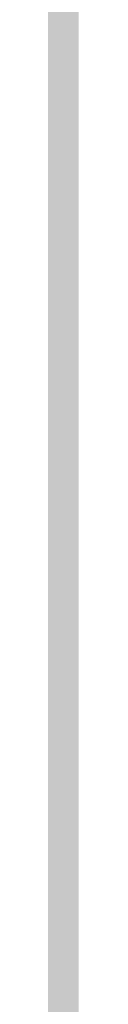
# Model space of a CAD drawing. Units: inches. Extents: x 2083 to 3317, y 1141 to 2115.
# Tile 181 of 256: x 3126.95825 to 3126.9594, y 1263.29018 to 1263.35483. Entities that reach past the tile are written whole.
import ezdxf

# ---------------------------------------------------------------- set-up
doc = ezdxf.new("R2010")
doc.units = ezdxf.units.IN
doc.layers.add('A-ANNO-DIMS', color=2, linetype='Continuous', lineweight=18)
doc.layers.add('A-WALL-PATT', color=251, linetype='Continuous', lineweight=13, true_color=0x636466)
doc.styles.get("Standard").update_dxf_attribs({"font": 'arial.ttf'})
doc.dimstyles.new('ISO-25', dxfattribs={"dimtxt": 12, "dimasz": 12, "dimexe": 1.25, "dimexo": 0.625, "dimtad": 1, "dimlunit": 3, "dimtxsty": 'Standard', "dimcen": 2.5, "dimadec": 0, "dimazin": 0, "dimtfac": 1, "dimtmove": 0, "dimatfit": 3, "dimfxl": 1, "dimarcsym": 0})

# ---------------------------------------------------------------- blocks, each defined once
blk = doc.blocks.new('*D26')
at = {"layer": 'A-ANNO-DIMS', "color": 0, "lineweight": -2, "transparency": 16777216}
for p, q in [((3088.985844, 1274.915092), (3088.985844, 1270.951963)), ((3111.240037, 1274.915092), (3111.240037, 1270.951963)), ((3076.985844, 1272.201963), (2840.262447, 1272.201963)), ((3111.240037, 1272.201963), (3088.985844, 1272.201963)), ((3123.240037, 1272.201963), (3135.240037, 1272.201963))]:
    blk.add_line(p, q, dxfattribs=at)
at = {"layer": 'A-ANNO-DIMS', "color": 0, "transparency": 16777216}
for points in [[(3076.985844, 1274.201963), (3076.985844, 1270.201963), (3088.985844, 1272.201963)], [(3123.240037, 1274.201963), (3123.240037, 1270.201963), (3111.240037, 1272.201963)]]:
    blk.add_solid(points, dxfattribs=at)
at = {"layer": 'Defpoints', "color": 0, "transparency": 16777216}
for p in [(3088.985844, 1275.540092), (3111.240037, 1275.540092), (3088.985844, 1272.201963)]:
    blk.add_point(p, dxfattribs=at)
at = {"layer": 'A-ANNO-DIMS', "color": 0, "transparency": 16777216, "insert": (2952.624146, 1279.031602), "char_height": 12, "attachment_point": 5}
blk.add_mtext('NIGHTSTAND 1\'-10 1/2" TYP.', dxfattribs=at)
blk = doc.blocks.new('*D27')
at = {"layer": 'A-ANNO-DIMS', "color": 0, "lineweight": -2, "transparency": 16777216}
for p, q in [((3114.578165, 1309.794285), (3114.578165, 1321.794285)), ((3111.865037, 1297.794285), (3115.828165, 1297.794285)), ((3114.578165, 1297.794285), (3114.578165, 1275.540092)), ((3111.865037, 1275.540092), (3115.828165, 1275.540092)), ((3114.578165, 1263.540092), (3114.578165, 1140.988591))]:
    blk.add_line(p, q, dxfattribs=at)
at = {"layer": 'A-ANNO-DIMS', "color": 0, "transparency": 16777216}
for points in [[(3112.578165, 1309.794285), (3116.578165, 1309.794285), (3114.578165, 1297.794285)], [(3112.578165, 1263.540092), (3116.578165, 1263.540092), (3114.578165, 1275.540092)]]:
    blk.add_solid(points, dxfattribs=at)
at = {"layer": 'Defpoints', "color": 0, "transparency": 16777216}
for p in [(3111.240037, 1297.794285), (3111.240037, 1275.540092), (3114.578165, 1275.540092)]:
    blk.add_point(p, dxfattribs=at)
at = {"layer": 'A-ANNO-DIMS', "color": 0, "transparency": 16777216, "insert": (3107.748527, 1196.264342), "char_height": 12, "attachment_point": 5, "rotation": 90}
blk.add_mtext('1\'-10 1/2" TYP.', dxfattribs=at)

msp = doc.modelspace()

# ---------------------------------------------------------------- hatches: boundary and pattern name
at = {"layer": 'A-WALL-PATT'}
h = msp.add_hatch(color=256, dxfattribs=at)
h.dxf.hatch_style = 1
h.paths.add_polyline_path([(3126.959783, 2020.76136), (2748.959783, 2020.76136), (2604.959783, 2020.76136), (2226.959783, 2020.76136), (2226.959783, 1702.76136), (2466.959783, 1702.76136), (2466.959783, 1582.76136), (2418.959783, 1582.76136), (2418.959783, 1477.76136), (2226.959783, 1477.76136), (2226.959783, 1263.26136), (2544.959783, 1263.26136), (2544.959783, 1411.76136), (2604.959783, 1411.76136), (2685.959783, 1411.76136), (2685.959783, 1420.76136), (2604.959783, 1420.76136), (2604.959783, 1573.76136), (2604.959783, 1702.76136), (2604.959783, 2011.76136), (2748.959783, 2011.76136), (2748.959783, 1702.76136), (2862.959783, 1702.76136), (2862.959783, 1621.76136), (2871.959783, 1621.76136), (2871.959783, 1702.76136), (2883.959783, 1702.76136), (2883.959783, 1706.939459, -0.026459), (2883.959783, 1711.76136), (2757.959783, 1711.76136), (2757.959783, 1807.76136), (2787.959783, 1807.76136), (2787.959783, 1812.26136), (2757.959783, 1812.26136), (2757.959783, 2011.76136), (2877.959783, 2011.76136), (2877.959783, 1812.26136), (2847.959783, 1812.26136), (2847.959783, 1807.76136), (2889.835742, 1807.76136), (2889.835742, 1812.26136), (2882.459783, 1812.26136), (2882.459783, 2011.76136), (3117.959783, 2011.76136), (3117.959783, 1812.26136), (2937.835742, 1812.26136), (2937.835742, 1807.76136), (2995.709783, 1807.76136), (2995.709783, 1796.117666), (3000.209783, 1796.117666), (3000.209783, 1807.76136), (3117.959783, 1807.76136), (3117.959783, 1711.76136), (3000.209783, 1711.76136), (3000.209783, 1760.117666), (2998.572705, 1760.117666, -0.020711), (2995.709783, 1760.117666), (2995.709783, 1711.76136), (2931.959783, 1711.76136), (2931.959783, 1702.76136), (3126.959783, 1702.76136)])
h.paths.add_polyline_path([(2471.459783, 2011.76136), (2471.459783, 1810.01136), (2462.716936, 1810.01136), (2462.716936, 1805.51136), (2505.959783, 1805.51136), (2505.959783, 1810.01136), (2475.959783, 1810.01136), (2475.959783, 2011.76136), (2595.959783, 2011.76136), (2595.959783, 1810.01136), (2565.959783, 1810.01136), (2565.959783, 1805.51136), (2595.959783, 1805.51136), (2595.959783, 1711.76136), (2235.959783, 1711.76136), (2235.959783, 1805.51136), (2353.709783, 1805.51136), (2353.709783, 1796.054162), (2358.209783, 1796.054162), (2358.209783, 1805.51136), (2414.716936, 1805.51136), (2414.716936, 1810.01136), (2235.959783, 1810.01136), (2235.959783, 2011.76136)], flags=16)
h.paths.add_polyline_path([(2270.204734, 1994.610008), (2270.204734, 1970.610008), (2246.204734, 1970.610008), (2246.204734, 1994.610008)], flags=0)
edge = h.paths.add_edge_path(flags=0)
edge.add_ellipse((2332.027391, 1899.798176), major_axis=(-3.042994, 3.042994), ratio=0.16825245, start_angle=-161.332166, end_angle=-156.307114, ccw=False)
edge.add_ellipse((2333.082037, 1898.74353), major_axis=(-1.054646, 1.054646), ratio=0.4535321, start_angle=-123.371019, end_angle=-94.159107)
edge = h.paths.add_edge_path(flags=0)
edge.add_ellipse((2332.027391, 1968.87629), major_axis=(3.042994, 3.042994), ratio=0.16825245, start_angle=18.667834, end_angle=23.692886)
edge.add_spline(control_points=[(2332.925596, 1970.691105), (2332.226768, 1970.3361), (2330.893709, 1969.658905), (2328.41308, 1970.932138), (2327.203934, 1967.748712), (2324.709596, 1969.955589), (2322.532822, 1967.012354), (2320.012846, 1971.295812), (2317.680308, 1968.157845), (2316.040526, 1967.102047), (2315.426904, 1966.809602)], knot_values=[0, 0, 0, 0, 2.267059, 4.324559, 6.685584, 8.878641, 11.121502, 14.300359, 17.755284, 19.732645, 19.732645, 19.732645, 19.732645], degree=3, periodic=0)
edge.add_ellipse((2332.027391, 1968.87629), major_axis=(3.042994, 3.042994), ratio=0.16825245, start_angle=18.667834, end_angle=23.692886, ccw=False)
edge.add_ellipse((2333.082037, 1969.930936), major_axis=(1.054646, 1.054646), ratio=0.4535321, start_angle=56.628981, end_angle=85.840893, ccw=False)
edge = h.paths.add_edge_path(flags=0)
edge.add_spline(control_points=[(2296.428287, 1967.987908), (2293.627804, 1965.336314), (2287.703624, 1959.727094), (2299.74386, 1949.995699), (2294.532591, 1935.668528), (2290.573228, 1920.603512), (2293.394124, 1909.973691), (2296.185407, 1904.966543)], knot_values=[0.099185, 0.099185, 0.099185, 0.099185, 0.345301, 0.619822, 0.982653, 1.386093, 1.810555, 1.810555, 1.810555, 1.810555], degree=3, periodic=0)
edge.add_spline(control_points=[(2296.185407, 1904.966543), (2297.383582, 1902.6193), (2298.000969, 1901.949312), (2298.55297, 1901.468155)], knot_values=[0.006246, 0.006246, 0.006246, 0.006246, 0.055476, 0.055476, 0.055476, 0.055476], degree=3, periodic=0)
edge.add_spline(control_points=[(2298.55297, 1901.468155), (2297.258612, 1900.923224), (2295.225294, 1900.232126), (2293.060229, 1900.614205), (2292.101423, 1900.788415), (2292.089578, 1900.790568)], knot_values=[0.312835, 0.312835, 0.312835, 0.312835, 0.40178, 0.474987, 0.475903, 0.475903, 0.475903, 0.475903], degree=3, periodic=0)
edge.add_arc((2292.793646, 1904.664109), 3.937008, 215.420897, 259.698179, ccw=False)
edge.add_spline(control_points=[(2289.585314, 1902.382304), (2289.476652, 1902.535087), (2289.36848, 1902.688035), (2289.260865, 1902.84117)], knot_values=[0.102872, 0.102872, 0.102872, 0.102872, 0.116896, 0.116896, 0.116896, 0.116896], degree=3, periodic=0)
edge.add_spline(control_points=[(2289.260865, 1902.84117), (2288.686604, 1902.550192), (2287.640048, 1902.019902), (2285.881337, 1901.873954), (2283.852972, 1901.504352), (2281.719987, 1899.710538), (2278.466991, 1899.492942), (2276.157136, 1901.883202), (2272.258953, 1899.804071), (2267.777605, 1901.843183), (2262.243882, 1900.184033), (2257.414927, 1901.782061), (2254.318374, 1900.72612), (2253.178285, 1900.337343)], knot_values=[0, 0, 0, 0, 1.907977, 3.477176, 5.261074, 7.972851, 11.680248, 13.717921, 16.939592, 22.789562, 27.502503, 33.595215, 37.145618, 37.145618, 37.145618, 37.145618], degree=3, periodic=0)
edge.add_line((2253.178285, 1900.337343), (2250.24424, 1902.84117))
edge.add_line((2250.24424, 1902.84117), (2250.24424, 1965.833296))
edge.add_line((2250.24424, 1965.833296), (2253.178285, 1968.337123))
edge.add_spline(control_points=[(2253.178285, 1968.337123), (2254.318374, 1967.948346), (2257.414927, 1966.892405), (2262.243882, 1968.490433), (2267.777605, 1966.831283), (2271.52673, 1968.537217), (2273.875914, 1967.828289), (2274.206701, 1967.727642)], knot_values=[0, 0, 0, 0, 0.09018, 0.244935, 0.364644, 0.513233, 0.537855, 0.537855, 0.537855, 0.537855], degree=3, periodic=0)
edge.add_arc((2274.352887, 1963.793349), 3.937008, 72.051134, 92.127949, ccw=False)
edge.add_arc((2281.296933, 1985.230003), 18.596298, 252.0511336, 288.5657217)
edge.add_arc((2292.316717, 1956.02888), 12.646081, 71.0267879, 113.7782184, ccw=False)
edge = h.paths.add_edge_path(flags=0)
edge.add_spline(control_points=[(2274.899415, 1951.856195), (2275.066156, 1951.616592), (2275.232687, 1951.376588), (2275.397987, 1951.135855)], knot_values=[1.409916, 1.409916, 1.409916, 1.409916, 1.43159, 1.43159, 1.43159, 1.43159], degree=3, periodic=0)
edge.add_spline(control_points=[(2275.397987, 1951.135855), (2275.792106, 1950.561885), (2276.179231, 1949.983774), (2276.545546, 1949.397103)], knot_values=[1.358238, 1.358238, 1.358238, 1.358238, 1.409916, 1.409916, 1.409916, 1.409916], degree=3, periodic=0)
edge.add_line((2276.545546, 1949.397103), (2277.437289, 1947.862185))
edge.add_spline(control_points=[(2277.437289, 1947.862185), (2276.303834, 1945.673115), (2274.639698, 1942.426882), (2274.631615, 1938.0939), (2272.799124, 1930.85155), (2274.356426, 1943.897046), (2275.947681, 1947.923356), (2276.545546, 1949.397103)], knot_values=[0.005632, 0.005632, 0.005632, 0.005632, 0.186014, 0.266002, 0.357087, 0.59639, 0.739732, 0.739732, 0.739732, 0.739732], degree=3, periodic=0)
edge.add_spline(control_points=[(2276.545546, 1949.397103), (2276.179231, 1949.983774), (2275.792106, 1950.561885), (2275.397987, 1951.135855)], knot_values=[1.358238, 1.358238, 1.358238, 1.358238, 1.409916, 1.409916, 1.409916, 1.409916], degree=3, periodic=0)
edge.add_spline(control_points=[(2275.397987, 1951.135855), (2274.9425, 1950.080452), (2274.20776, 1948.025272), (2273.934602, 1944.851477), (2272.468534, 1937.627489), (2273.466216, 1945.696466), (2274.700615, 1951.059472), (2274.899415, 1951.856195)], knot_values=[0.104364, 0.104364, 0.104364, 0.104364, 0.189636, 0.269624, 0.36071, 0.600013, 0.644622, 0.644622, 0.644622, 0.644622], degree=3, periodic=0)
h.paths.add_polyline_path([(2269.167514, 1963.127573, -0.357527), (2268.170633, 1960.97637, -0.092561), (2268.170633, 1939.436325, -0.357527), (2269.167514, 1937.285122, -0.357527), (2267.01631, 1938.282002, -0.164785), (2254.685581, 1938.282002, -0.357527), (2252.534378, 1937.285122, -0.357527), (2253.531259, 1939.436325, -0.092561), (2253.531259, 1960.97637, -0.357527), (2252.534378, 1963.127573, -0.357527), (2254.685581, 1962.130692, -0.164785), (2267.01631, 1962.130692, -0.357527)], flags=0)
h.paths.add_polyline_path([(2248.874068, 1967.8018), (2248.874068, 1957.02771), (2249.457783, 1957.02771), (2249.457783, 1911.646756), (2248.874068, 1911.646756), (2248.874068, 1900.872666), (2246.511863, 1900.872666, 0.197327), (2244.149658, 1902.456873), (2244.149658, 1966.217592, 0.197327), (2246.511863, 1967.8018)], flags=0)
h.paths.add_polyline_path([(2269.167514, 1931.389344, -0.357527), (2268.170633, 1929.238141, -0.092561), (2268.170633, 1907.698096, -0.357527), (2269.167514, 1905.546893, -0.357527), (2267.01631, 1906.543774, -0.164785), (2254.685581, 1906.543774, -0.357527), (2252.534378, 1905.546893, -0.357527), (2253.531259, 1907.698096, -0.092561), (2253.531259, 1929.238141, -0.357527), (2252.534378, 1931.389344, -0.357527), (2254.685581, 1930.392463, -0.164785), (2267.01631, 1930.392463, -0.357527)], flags=0)
edge = h.paths.add_edge_path(flags=0)
edge.add_spline(control_points=[(2276.196858, 1906.723702), (2276.168144, 1909.028928), (2276.114049, 1913.371852), (2270.598417, 1924.924978), (2273.905175, 1919.012779), (2275.921711, 1916.262063), (2275.47457, 1912.402149), (2277.257874, 1910.380621), (2276.696044, 1908.225036), (2276.646218, 1906.813023), (2276.617825, 1906.008407)], knot_values=[0, 0, 0, 0, 8.61026, 16.221274, 18.843057, 23.804898, 27.440828, 29.356102, 31.203478, 33.650687, 33.650687, 33.650687, 33.650687], degree=3, periodic=0)
edge.add_spline(control_points=[(2276.617825, 1906.008407), (2276.623313, 1905.624144), (2276.497738, 1904.628661), (2275.441779, 1903.854725), (2274.937314, 1903.08045), (2274.85908, 1902.84117)], knot_values=[0.156488, 0.156488, 0.156488, 0.156488, 0.184398, 0.231376, 0.250598, 0.250598, 0.250598, 0.250598], degree=3, periodic=0)
edge.add_line((2274.85908, 1902.84117), (2276.50598, 1902.84117))
edge.add_spline(control_points=[(2276.50598, 1902.84117), (2276.788308, 1903.08494), (2277.665071, 1904.125196), (2278.249538, 1904.340738), (2277.653872, 1908.527387), (2278.15567, 1906.227808), (2278.100464, 1905.285948), (2278.846675, 1904.069005), (2277.856785, 1903.414948), (2277.874191, 1902.99105), (2277.903562, 1902.84117)], knot_values=[0.059574, 0.059574, 0.059574, 0.059574, 0.080753, 0.103741, 0.16972, 0.176036, 0.207137, 0.240474, 0.262341, 0.27366, 0.27366, 0.27366, 0.27366], degree=3, periodic=0)
edge.add_line((2277.903562, 1902.84117), (2280.029825, 1902.84117))
edge.add_spline(control_points=[(2280.029825, 1902.84117), (2279.888221, 1903.088398), (2279.499257, 1903.981551), (2280.152284, 1905.939349), (2278.103615, 1909.657757), (2279.762395, 1907.185285), (2280.3279, 1904.874861), (2280.485109, 1903.48959), (2281.463269, 1903.249432), (2281.758343, 1902.936497), (2281.834036, 1902.84117)], knot_values=[0.013856, 0.013856, 0.013856, 0.013856, 0.034874, 0.088867, 0.107879, 0.126738, 0.158714, 0.193757, 0.217487, 0.226722, 0.226722, 0.226722, 0.226722], degree=3, periodic=0)
edge.add_spline(control_points=[(2281.834036, 1902.84117), (2281.787535, 1902.826703), (2281.647022, 1902.782988), (2281.395527, 1902.85949), (2281.088077, 1902.985242), (2280.720683, 1903.060902), (2280.333451, 1903.025726), (2280.124767, 1902.898879), (2280.029825, 1902.84117)], knot_values=[0, 0, 0, 0, 0.14413, 0.435517, 0.749276, 1.153046, 1.548371, 1.878348, 1.878348, 1.878348, 1.878348], degree=3, periodic=0)
edge.add_line((2280.029825, 1902.84117), (2277.903562, 1902.84117))
edge.add_spline(control_points=[(2277.903562, 1902.84117), (2277.892855, 1902.795855), (2277.865396, 1902.679637), (2277.607479, 1902.687483), (2277.27405, 1902.8007), (2276.837921, 1902.619775), (2276.583807, 1902.789261), (2276.50598, 1902.84117)], knot_values=[0, 0, 0, 0, 0.127189, 0.326199, 0.628009, 1.24357, 1.515331, 1.515331, 1.515331, 1.515331], degree=3, periodic=0)
edge.add_line((2276.50598, 1902.84117), (2274.85908, 1902.84117))
edge.add_spline(control_points=[(2274.85908, 1902.84117), (2274.814437, 1902.898587), (2274.72513, 1903.013446), (2274.493477, 1903.118968), (2274.244285, 1902.960539), (2273.937121, 1903.184942), (2273.614039, 1902.983143), (2273.408316, 1902.883045), (2273.322254, 1902.84117)], knot_values=[0, 0, 0, 0, 0.21843, 0.436957, 0.687977, 0.990379, 1.398396, 1.69185, 1.69185, 1.69185, 1.69185], degree=3, periodic=0)
edge.add_spline(control_points=[(2273.322254, 1902.84117), (2273.61674, 1903.445692), (2274.273998, 1904.538253), (2276.027239, 1904.573702), (2276.206963, 1906.583637), (2276.196858, 1906.723702)], knot_values=[0.012227, 0.012227, 0.012227, 0.012227, 0.059472, 0.106218, 0.134458, 0.134458, 0.134458, 0.134458], degree=3, periodic=0)
h.paths.add_polyline_path([(2270.776054, 1897.789828), (2270.776054, 1873.789828), (2246.776054, 1873.789828), (2246.776054, 1897.789828)], flags=0)
h.paths.add_polyline_path([(2353.709783, 1760.005059), (2353.709783, 1760.054162), (2358.209783, 1760.054162, -0.033729)], flags=0)
h.paths.add_polyline_path([(2321.819119, 1737.529186), (2341.995327, 1737.529186, -0.414214), (2343.203273, 1736.321241), (2343.203273, 1721.020596, -0.414214), (2341.995327, 1719.812651), (2321.819119, 1719.812651, -0.414214), (2320.611173, 1721.020596), (2320.611173, 1736.321241, -0.414214)], flags=0)
h.paths.add_polyline_path([(2324.23501, 1736.321241), (2339.579436, 1736.321241, -0.414214), (2341.995327, 1733.905349), (2341.995327, 1725.44973, -0.414214), (2339.579436, 1723.033839), (2333.680588, 1723.033839), (2333.845317, 1722.045467, -0.870646), (2335.425399, 1721.825893, -0.767327), (2333.922694, 1721.423245), (2331.291024, 1721.423245, -0.767327), (2329.788319, 1721.825893, -0.870646), (2331.368401, 1722.045467), (2331.53313, 1723.033839), (2324.23501, 1723.033839, -0.414214), (2321.819119, 1725.44973), (2321.819119, 1733.905349, -0.414214)], flags=0)
h.paths.add_polyline_path([(2570.483789, 1928.615444), (2589.683789, 1928.615444), (2590.168829, 1928.615444), (2590.168829, 1904.993397), (2570.483789, 1904.993397)], flags=0)
h.paths.add_polyline_path([(2574.447324, 1927.263822, -1), (2572.828836, 1927.263822, -1)], flags=0)
h.paths.add_polyline_path([(2573.089867, 1926.940877), (2573.925032, 1927.776042), (2574.147743, 1927.553332), (2573.312577, 1926.718166)], flags=0)
h.paths.add_polyline_path([(2578.779065, 1919.729618, -1), (2571.591663, 1919.729618, -1)], flags=0)
h.paths.add_polyline_path([(2578.385364, 1919.729618, -1), (2571.985364, 1919.729618, -1)], flags=0)
h.paths.add_polyline_path([(2331.595764, 1729.476216, -1), (2333.617954, 1729.476216, -1)], flags=0)
h.paths.add_polyline_path([(2578.034228, 1927.263822, -1), (2576.41574, 1927.263822, -1)], flags=0)
h.paths.add_polyline_path([(2576.688851, 1927.531089), (2576.911562, 1927.753799), (2577.746728, 1926.918634), (2577.524017, 1926.695923)], flags=0)
h.paths.add_polyline_path([(2578.139065, 1909.859539, -1), (2572.231663, 1909.859539, -1)], flags=0)
h.paths.add_polyline_path([(2577.745364, 1909.859539, -1), (2572.625364, 1909.859539, -1)], flags=0)
h.paths.add_polyline_path([(2583.797718, 1927.263822, -1), (2582.179229, 1927.263822, -1)], flags=0)
h.paths.add_polyline_path([(2582.718649, 1927.753799), (2583.553814, 1926.918634), (2583.331103, 1926.695923), (2582.495938, 1927.531089)], flags=0)
h.paths.add_polyline_path([(2582.495938, 1927.531089), (2582.718649, 1927.753799), (2583.553814, 1926.918634), (2583.331103, 1926.695923)], flags=0)
h.paths.add_polyline_path([(2587.739065, 1920.529618, -1), (2581.831663, 1920.529618, -1)], flags=0)
h.paths.add_polyline_path([(2587.345364, 1920.529618, -1), (2582.225364, 1920.529618, -1)], flags=0)
h.paths.add_polyline_path([(2587.384622, 1927.263822, -1), (2585.766133, 1927.263822, -1)], flags=0)
h.paths.add_polyline_path([(2586.081993, 1926.980247), (2586.917158, 1927.815412), (2587.139869, 1927.592702), (2586.304703, 1926.757536)], flags=0)
h.paths.add_polyline_path([(2588.379065, 1910.659539, -1), (2581.191663, 1910.659539, -1)], flags=0)
h.paths.add_polyline_path([(2587.985364, 1910.659539, -1), (2581.585364, 1910.659539, -1)], flags=0)
h.paths.add_polyline_path([(2417.167729, 1729.477895), (2437.343937, 1729.477895, -0.414214), (2438.551883, 1728.26995), (2438.551883, 1712.969306, -0.414214), (2437.343937, 1711.76136), (2417.167729, 1711.76136, -0.414214), (2415.959783, 1712.969306), (2415.959783, 1728.26995, -0.414214)], flags=0)
h.paths.add_polyline_path([(2419.58362, 1728.26995), (2434.928046, 1728.26995, -0.414214), (2437.343937, 1725.854059), (2437.343937, 1717.39844, -0.414214), (2434.928046, 1714.982548), (2429.029199, 1714.982548), (2429.193927, 1713.994176, -0.870646), (2430.774009, 1713.774603, -0.767327), (2429.271304, 1713.371954), (2426.639634, 1713.371954, -0.767327), (2425.136929, 1713.774603, -0.870646), (2426.717011, 1713.994176), (2426.88174, 1714.982548), (2419.58362, 1714.982548, -0.414214), (2417.167729, 1717.39844), (2417.167729, 1725.854059, -0.414214)], flags=0)
h.paths.add_polyline_path([(2419.58362, 1728.26995), (2434.928046, 1728.26995, -0.414214), (2437.343937, 1725.854059), (2437.343937, 1717.39844, -0.414214), (2434.928046, 1714.982548), (2429.029199, 1714.982548), (2428.358118, 1719.009034), (2427.552821, 1719.009034), (2426.88174, 1714.982548), (2419.58362, 1714.982548, -0.414214), (2417.167729, 1717.39844), (2417.167729, 1725.854059, -0.414214)], flags=0)
h.paths.add_polyline_path([(2426.944374, 1721.424925, -1), (2428.966564, 1721.424925, -1)], flags=0)
h.paths.add_polyline_path([(2475.959783, 1702.76136), (2595.959783, 1702.76136), (2595.959783, 1582.76136), (2475.959783, 1582.76136)], flags=16)
h.paths.add_polyline_path([(2427.959783, 1573.76136), (2595.959783, 1573.76136), (2595.959783, 1468.76136), (2595.959783, 1420.76136), (2384.459783, 1420.76136), (2384.459783, 1468.76136), (2427.959783, 1468.76136)], flags=16)
h.paths.add_polyline_path([(2379.959783, 1468.76136), (2379.959783, 1420.76136), (2235.959783, 1420.76136), (2235.959783, 1468.76136)], flags=16)
h.paths.add_polyline_path([(2317.815996, 1466.695767), (2337.992205, 1466.695767, -0.414214), (2339.20015, 1465.487821), (2339.20015, 1450.187177, -0.414214), (2337.992205, 1448.979232), (2317.815996, 1448.979232, -0.414214), (2316.608051, 1450.187177), (2316.608051, 1465.487821, -0.414214)], flags=0)
h.paths.add_polyline_path([(2320.231887, 1465.487821), (2335.576313, 1465.487821, -0.414214), (2337.992205, 1463.07193), (2337.992205, 1454.616311, -0.414214), (2335.576313, 1452.20042), (2329.677466, 1452.20042), (2329.842195, 1451.212047, -0.870646), (2331.422276, 1450.992474, -0.767327), (2329.919571, 1450.589826), (2327.287902, 1450.589826, -0.767327), (2325.785197, 1450.992474, -0.870646), (2327.365278, 1451.212047), (2327.530007, 1452.20042), (2320.231887, 1452.20042, -0.414214), (2317.815996, 1454.616311), (2317.815996, 1463.07193, -0.414214)], flags=0)
h.paths.add_polyline_path([(2320.231887, 1465.487821), (2335.576313, 1465.487821, -0.414214), (2337.992205, 1463.07193), (2337.992205, 1454.616311, -0.414214), (2335.576313, 1452.20042), (2329.677466, 1452.20042), (2329.006385, 1456.226905), (2328.201088, 1456.226905), (2327.530007, 1452.20042), (2320.231887, 1452.20042, -0.414214), (2317.815996, 1454.616311), (2317.815996, 1463.07193, -0.414214)], flags=0)
h.paths.add_polyline_path([(2327.592641, 1458.642796, -1), (2329.614832, 1458.642796, -1)], flags=0)
h.paths.add_polyline_path([(2244.411744, 1433.340453), (2241.920945, 1433.340453, -0.414214), (2240.017856, 1435.243542), (2240.017856, 1440.952808, -0.414211), (2241.920925, 1442.855897), (2244.411744, 1442.855897, -1.976472)], flags=0)
h.paths.add_polyline_path([(2245.356888, 1434.397536, -0.414214), (2245.356888, 1441.798814, -2.144098)], flags=0)
h.paths.add_polyline_path([(2535.959783, 1416.26136), (2535.959783, 1272.26136), (2235.959783, 1272.26136), (2235.959783, 1416.26136)], flags=16)
h.paths.add_polyline_path([(2260.119561, 1384.292841), (2260.119561, 1362.038649), (2237.865369, 1362.038649), (2237.865369, 1384.292841)], flags=0)
edge = h.paths.add_edge_path(flags=0)
edge.add_line((2318.251847, 1362.093298), (2318.145797, 1362.000973))
edge.add_ellipse((2317.445116, 1360.431044), major_axis=(2.82164, 2.82164), ratio=0.16825245, start_angle=18.667834, end_angle=20.948127, ccw=False)
edge.add_ellipse((2318.423045, 1361.408974), major_axis=(0.977929, 0.977929), ratio=0.4535321, start_angle=56.628981, end_angle=70.226201, ccw=False)
edge = h.paths.add_edge_path(flags=0)
edge.add_line((2319.10737, 1295.571078), (2319.015044, 1295.677128))
edge.add_ellipse((2317.445116, 1296.377809), major_axis=(-2.82164, 2.82164), ratio=0.16825245, start_angle=-161.332166, end_angle=-159.051873, ccw=False)
edge.add_ellipse((2318.423045, 1295.39988), major_axis=(-0.977929, 0.977929), ratio=0.4535321, start_angle=-123.371019, end_angle=-109.773799)
edge = h.paths.add_edge_path(flags=0)
edge.add_spline(control_points=[(2284.210349, 1301.170219), (2284.580688, 1300.444719), (2284.891189, 1299.892024), (2285.159553, 1299.461018)], knot_values=[0.039066, 0.039066, 0.039066, 0.039066, 0.055476, 0.055476, 0.055476, 0.055476], degree=3, periodic=0)
edge.add_line((2285.159553, 1299.461018), (2284.210349, 1301.170219))
edge = h.paths.add_edge_path(flags=0)
edge.add_line((2280.412458, 1297.298013), (2283.369991, 1297.036122))
edge.add_line((2283.369991, 1297.036122), (2286.40569, 1297.92631))
edge.add_spline(control_points=[(2286.40569, 1297.92631), (2285.305487, 1297.463119), (2284.344777, 1297.129151), (2283.369991, 1297.036122)], knot_values=[0.394369, 0.394369, 0.394369, 0.394369, 0.475903, 0.475903, 0.475903, 0.475903], degree=3, periodic=0)
edge.add_spline(control_points=[(2283.369991, 1297.036122), (2283.28139, 1297.027666), (2282.316289, 1296.957336), (2281.312502, 1297.134479), (2280.423441, 1297.296016), (2280.412458, 1297.298013)], knot_values=[0.312835, 0.312835, 0.312835, 0.312835, 0.320246, 0.393453, 0.394369, 0.394369, 0.394369, 0.394369], degree=3, periodic=0)
edge = h.paths.add_edge_path(flags=0)
edge.add_line((2284.435561, 1359.607285), (2280.446291, 1355.328047))
edge.add_line((2280.446291, 1355.328047), (2279.579987, 1351.017754))
edge.add_line((2279.579987, 1351.017754), (2282.412974, 1346.580433))
edge.add_spline(control_points=[(2282.412974, 1346.580433), (2283.153331, 1345.589236), (2284.252896, 1344.028897), (2284.801037, 1342.387167), (2284.935162, 1341.805544)], knot_values=[1.240098, 1.240098, 1.240098, 1.240098, 1.332892, 1.382712, 1.382712, 1.382712, 1.382712], degree=3, periodic=0)
edge.add_spline(control_points=[(2284.935162, 1341.805544), (2285.319108, 1340.1406), (2285.233029, 1338.409204), (2284.909938, 1336.654122)], knot_values=[1.097484, 1.097484, 1.097484, 1.097484, 1.240098, 1.240098, 1.240098, 1.240098], degree=3, periodic=0)
edge.add_spline(control_points=[(2284.909938, 1336.654122), (2284.586848, 1334.89904), (2284.026745, 1333.120272), (2283.462644, 1331.360585)], knot_values=[0.95487, 0.95487, 0.95487, 0.95487, 1.097484, 1.097484, 1.097484, 1.097484], degree=3, periodic=0)
edge.add_line((2283.462644, 1331.360585), (2281.890376, 1326.153357))
edge.add_line((2281.890376, 1326.153357), (2280.756259, 1321.056089))
edge.add_line((2280.756259, 1321.056089), (2280.299205, 1316.001977))
edge.add_line((2280.299205, 1316.001977), (2280.715933, 1310.950068))
edge.add_line((2280.715933, 1310.950068), (2282.028094, 1305.972137))
edge.add_line((2282.028094, 1305.972137), (2284.210349, 1301.170219))
edge.add_spline(control_points=[(2284.210349, 1301.170219), (2283.340731, 1302.730185), (2282.611904, 1304.336493), (2282.028094, 1305.972137)], knot_values=[0.099185, 0.099185, 0.099185, 0.099185, 0.241799, 0.241799, 0.241799, 0.241799], degree=3, periodic=0)
edge.add_spline(control_points=[(2282.028094, 1305.972137), (2281.444283, 1307.60778), (2281.005489, 1309.272759), (2280.715933, 1310.950068)], knot_values=[0.241799, 0.241799, 0.241799, 0.241799, 0.384413, 0.384413, 0.384413, 0.384413], degree=3, periodic=0)
edge.add_spline(control_points=[(2280.715933, 1310.950068), (2280.433241, 1312.587613), (2280.289386, 1314.276959), (2280.298894, 1315.962032), (2280.299205, 1316.001977)], knot_values=[0.384413, 0.384413, 0.384413, 0.384413, 0.523647, 0.527028, 0.527028, 0.527028, 0.527028], degree=3, periodic=0)
edge.add_spline(control_points=[(2280.299205, 1316.001977), (2280.312326, 1317.686955), (2280.477871, 1319.367926), (2280.756259, 1321.056089)], knot_values=[0.527028, 0.527028, 0.527028, 0.527028, 0.669642, 0.669642, 0.669642, 0.669642], degree=3, periodic=0)
edge.add_spline(control_points=[(2280.756259, 1321.056089), (2281.034648, 1322.744252), (2281.42588, 1324.439608), (2281.890376, 1326.153357)], knot_values=[0.669642, 0.669642, 0.669642, 0.669642, 0.812256, 0.812256, 0.812256, 0.812256], degree=3, periodic=0)
edge.add_spline(control_points=[(2281.890376, 1326.153357), (2282.264383, 1327.533251), (2282.78787, 1329.26181), (2283.352751, 1331.01778), (2283.462644, 1331.360585)], knot_values=[0.812256, 0.812256, 0.812256, 0.812256, 0.927087, 0.95487, 0.95487, 0.95487, 0.95487], degree=3, periodic=0)
edge.add_line((2283.462644, 1331.360585), (2284.909938, 1336.654122))
edge.add_line((2284.909938, 1336.654122), (2284.935162, 1341.805544))
edge.add_line((2284.935162, 1341.805544), (2282.412974, 1346.580433))
edge.add_spline(control_points=[(2282.412974, 1346.580433), (2281.275127, 1348.103792), (2280.078447, 1349.570318), (2279.579987, 1351.017754)], knot_values=[1.382712, 1.382712, 1.382712, 1.382712, 1.525326, 1.525326, 1.525326, 1.525326], degree=3, periodic=0)
edge.add_spline(control_points=[(2279.579987, 1351.017754), (2279.443282, 1351.414721), (2279.136312, 1352.856922), (2279.73519, 1354.290385), (2280.446291, 1355.328047)], knot_values=[1.525326, 1.525326, 1.525326, 1.525326, 1.564439, 1.667941, 1.667941, 1.667941, 1.667941], degree=3, periodic=0)
edge.add_spline(control_points=[(2280.446291, 1355.328047), (2281.426113, 1356.757835), (2282.930837, 1358.18256), (2284.435561, 1359.607285)], knot_values=[1.667941, 1.667941, 1.667941, 1.667941, 1.810555, 1.810555, 1.810555, 1.810555], degree=3, periodic=0)
edge.add_arc((2280.623075, 1348.518181), 11.72618, 71.0267879, 113.7782184)
edge.add_arc((2270.404892, 1375.595156), 17.243567, 252.0511336, 288.5657217, ccw=False)
edge.add_arc((2263.965969, 1355.717847), 3.650622, 72.051134, 92.127949)
edge.add_arc((2263.965969, 1355.717847), 3.650622, 92.127949, 177.98513)
edge.add_spline(control_points=[(2260.317604, 1355.846199), (2260.260417, 1354.220668), (2260.551278, 1350.186547), (2262.999344, 1346.766251), (2264.472741, 1344.649024)], knot_values=[1.43159, 1.43159, 1.43159, 1.43159, 1.564144, 1.770695, 1.770695, 1.770695, 1.770695], degree=3, periodic=0)
edge.add_line((2264.472741, 1344.649024), (2264.93559, 1343.98253))
edge.add_spline(control_points=[(2263.801044, 1340.248105), (2263.843238, 1340.514088), (2264.067244, 1341.756465), (2264.512693, 1343.002453), (2264.935047, 1343.981083)], knot_values=[0.53657, 0.53657, 0.53657, 0.53657, 0.559349, 0.644622, 0.644622, 0.644622, 0.644622], degree=3, periodic=0)
edge.add_spline(control_points=[(2264.935047, 1343.981083), (2265.117771, 1343.714975), (2265.298875, 1343.447906), (2265.476756, 1343.179365)], knot_values=[1.384077, 1.384077, 1.384077, 1.384077, 1.409916, 1.409916, 1.409916, 1.409916], degree=3, periodic=0)
edge.add_spline(control_points=[(2265.476756, 1343.179365), (2265.654637, 1342.910823), (2265.829296, 1342.64081), (2265.99913, 1342.368812)], knot_values=[1.358238, 1.358238, 1.358238, 1.358238, 1.384077, 1.384077, 1.384077, 1.384077], degree=3, periodic=0)
edge.add_line((2265.99913, 1342.368812), (2266.826006, 1340.945547))
edge.add_spline(control_points=[(2266.826006, 1340.945547), (2268.894401, 1337.089691), (2271.398173, 1325.843001), (2270.516164, 1310.568557), (2275.919376, 1301.860609), (2277.789511, 1299.19945)], knot_values=[0.116896, 0.116896, 0.116896, 0.116896, 0.472987, 1.050969, 1.313793, 1.313793, 1.313793, 1.313793], degree=3, periodic=0)
edge.add_spline(control_points=[(2277.789511, 1299.19945), (2277.839405, 1299.128452), (2277.889428, 1299.057498), (2277.939572, 1298.986584)], knot_values=[0.109884, 0.109884, 0.109884, 0.109884, 0.116896, 0.116896, 0.116896, 0.116896], degree=3, periodic=0)
edge.add_line((2277.939572, 1298.986584), (2277.788849, 1299.199114))
edge.add_spline(control_points=[(2277.788849, 1299.199114), (2277.256582, 1298.929414), (2276.28635, 1298.437902), (2275.039352, 1298.334419), (2274.38333, 1298.238895), (2274.215254, 1298.209338)], knot_values=[33.12187, 33.12187, 33.12187, 33.12187, 35.029056, 36.598255, 37.144827, 37.144827, 37.144827, 37.144827], degree=3, periodic=0)
edge.add_line((2274.215254, 1298.209338), (2273.073147, 1297.892961))
edge.add_spline(control_points=[(2273.073147, 1297.892961), (2272.322936, 1297.579784), (2271.039151, 1296.510508), (2269.248395, 1296.226062), (2268.4231, 1296.374654)], knot_values=[26.532584, 26.532584, 26.532584, 26.532584, 29.198919, 31.839101, 31.839101, 31.839101, 31.839101], degree=3, periodic=0)
edge.add_line((2268.4231, 1296.374654), (2263.878501, 1297.457534))
edge.add_spline(control_points=[(2263.878501, 1297.457534), (2263.556077, 1297.359435), (2261.860306, 1296.838694), (2260.23878, 1297.282407), (2258.933454, 1297.516461)], knot_values=[15.919551, 15.919551, 15.919551, 15.919551, 16.939592, 21.226067, 21.226067, 21.226067, 21.226067], degree=3, periodic=0)
edge.add_line((2258.933454, 1297.516461), (2254.055233, 1297.32901))
edge.add_spline(control_points=[(2254.055233, 1297.32901), (2253.755525, 1297.295815), (2252.113683, 1297.165174), (2250.461869, 1297.544221), (2249.129686, 1297.667882)], knot_values=[5.306517, 5.306517, 5.306517, 5.306517, 6.276435, 10.613034, 10.613034, 10.613034, 10.613034], degree=3, periodic=0)
edge.add_line((2249.129686, 1297.667882), (2244.33165, 1296.877756))
edge.add_line((2244.33165, 1296.877756), (2241.611033, 1299.19945))
edge.add_line((2241.611033, 1299.19945), (2241.611033, 1357.609404))
edge.add_line((2241.611033, 1357.609404), (2244.33165, 1359.931097))
edge.add_line((2244.33165, 1359.931097), (2252.728823, 1359.542692))
edge.add_spline(control_points=[(2252.728823, 1359.542692), (2252.870939, 1359.54644), (2253.30574, 1359.548172), (2253.739845, 1359.514274), (2254.031742, 1359.482426)], knot_values=[0.233291, 0.233291, 0.233291, 0.233291, 0.244935, 0.268927, 0.268927, 0.268927, 0.268927], degree=3, periodic=0)
edge.add_line((2254.031742, 1359.482426), (2259.58719, 1359.41639))
edge.add_spline(control_points=[(2259.58719, 1359.41639), (2260.677068, 1359.628503), (2262.073197, 1359.897003), (2263.523692, 1359.459278), (2263.830417, 1359.365952)], knot_values=[0.422516, 0.422516, 0.422516, 0.422516, 0.513233, 0.537855, 0.537855, 0.537855, 0.537855], degree=3, periodic=0)
edge.add_arc((2263.965969, 1355.717847), 3.650622, 72.051134, 92.127949, ccw=False)
edge.add_arc((2270.404892, 1375.595156), 17.243567, 252.0511336, 288.5657217)
edge.add_arc((2280.623075, 1348.518181), 11.72618, 71.0267879, 113.7782184, ccw=False)
h.paths.add_polyline_path([(2240.34053, 1359.434715), (2240.34053, 1349.444353), (2240.881785, 1349.444353), (2240.881785, 1307.3645), (2240.34053, 1307.3645), (2240.34053, 1297.374138), (2238.150157, 1297.374138, 0.197327), (2235.959783, 1298.843108), (2235.959783, 1357.965746, 0.197327), (2238.150157, 1359.434715)], flags=0)
h.paths.add_polyline_path([(2259.15779, 1355.1005, -0.357527), (2258.233425, 1353.10578, -0.092561), (2258.233425, 1333.132601, -0.357527), (2259.15779, 1331.13788, -0.357527), (2257.16307, 1332.062246, -0.164785), (2245.729302, 1332.062246, -0.357527), (2243.734582, 1331.13788, -0.357527), (2244.658947, 1333.132601, -0.092561), (2244.658947, 1353.10578, -0.357527), (2243.734582, 1355.1005, -0.357527), (2245.729302, 1354.176135, -0.164785), (2257.16307, 1354.176135, -0.357527)], flags=0)
edge = h.paths.add_edge_path(flags=0)
edge.add_line((2265.99913, 1342.368812), (2266.826006, 1340.945547))
edge.add_line((2266.826006, 1340.945547), (2265.307557, 1337.814066))
edge.add_line((2265.307557, 1337.814066), (2264.358232, 1334.652939))
edge.add_line((2264.358232, 1334.652939), (2264.262012, 1333.799705))
edge.add_spline(control_points=[(2264.262012, 1333.799705), (2264.208357, 1333.187055), (2264.16206, 1332.365525), (2264.007144, 1331.413933), (2263.969049, 1331.201834)], knot_values=[0.464444, 0.464444, 0.464444, 0.464444, 0.516691, 0.531608, 0.531608, 0.531608, 0.531608], degree=3, periodic=0)
edge.add_spline(control_points=[(2263.969049, 1331.201834), (2263.774535, 1330.118873), (2263.42437, 1328.790839), (2263.25742, 1328.530652), (2263.234028, 1328.514612)], knot_values=[0.372682, 0.372682, 0.372682, 0.372682, 0.44885, 0.464444, 0.464444, 0.464444, 0.464444], degree=3, periodic=0)
edge.add_spline(control_points=[(2263.234028, 1328.514612), (2263.096382, 1328.420227), (2263.13117, 1329.301477), (2263.274953, 1330.615749)], knot_values=[0.280919, 0.280919, 0.280919, 0.280919, 0.372682, 0.372682, 0.372682, 0.372682], degree=3, periodic=0)
edge.add_spline(control_points=[(2263.274953, 1330.615749), (2263.418736, 1331.930022), (2263.671515, 1333.677318), (2263.969852, 1335.315027)], knot_values=[0.189157, 0.189157, 0.189157, 0.189157, 0.280919, 0.280919, 0.280919, 0.280919], degree=3, periodic=0)
edge.add_spline(control_points=[(2263.969852, 1335.315027), (2264.100496, 1336.032192), (2264.418783, 1337.621911), (2264.754848, 1338.86443), (2264.947419, 1339.491124)], knot_values=[0.097394, 0.097394, 0.097394, 0.097394, 0.137578, 0.189157, 0.189157, 0.189157, 0.189157], degree=3, periodic=0)
edge.add_spline(control_points=[(2264.947419, 1339.491124), (2265.290017, 1340.606055), (2265.644238, 1341.493996), (2265.99913, 1342.368812)], knot_values=[0.005632, 0.005632, 0.005632, 0.005632, 0.097394, 0.097394, 0.097394, 0.097394], degree=3, periodic=0)
h.paths.add_polyline_path([(2259.15779, 1325.670973, -0.357527), (2258.233425, 1323.676253, -0.092561), (2258.233425, 1303.703073, -0.357527), (2259.15779, 1301.708353, -0.357527), (2257.16307, 1302.632719, -0.164785), (2245.729302, 1302.632719, -0.357527), (2243.734582, 1301.708353, -0.357527), (2244.658947, 1303.703073, -0.092561), (2244.658947, 1323.676253, -0.357527), (2243.734582, 1325.670973, -0.357527), (2245.729302, 1324.746608, -0.164785), (2257.16307, 1324.746608, -0.357527)], flags=0)
edge = h.paths.add_edge_path(flags=0)
edge.add_spline(control_points=[(2261.708938, 1317.311421), (2261.679482, 1317.41758), (2261.761858, 1317.388535), (2262.490736, 1316.089873), (2262.962185, 1315.300897)], knot_values=[14.955861, 14.955861, 14.955861, 14.955861, 16.221274, 18.694826, 18.694826, 18.694826, 18.694826], degree=3, periodic=0)
edge.add_spline(control_points=[(2262.962185, 1315.300897), (2262.990437, 1315.253617), (2263.702096, 1314.067376), (2264.348983, 1313.127153), (2264.730054, 1312.164154)], knot_values=[18.694826, 18.694826, 18.694826, 18.694826, 18.843057, 22.433791, 22.433791, 22.433791, 22.433791], degree=3, periodic=0)
edge.add_spline(control_points=[(2264.730054, 1312.164154), (2264.875565, 1311.796437), (2265.176873, 1310.769807), (2265.143069, 1309.559262), (2265.247736, 1308.824193)], knot_values=[22.433791, 22.433791, 22.433791, 22.433791, 23.804898, 26.172756, 26.172756, 26.172756, 26.172756], degree=3, periodic=0)
edge.add_line((2265.247736, 1308.824193), (2265.850774, 1307.171888))
edge.add_spline(control_points=[(2265.850774, 1307.171888), (2266.065025, 1306.821678), (2266.384387, 1306.332246), (2266.4244, 1305.780549), (2266.420369, 1305.611216)], knot_values=[28.062562, 28.062562, 28.062562, 28.062562, 29.356102, 29.911721, 29.911721, 29.911721, 29.911721], degree=3, periodic=0)
edge.add_spline(control_points=[(2266.420369, 1305.611216), (2266.416116, 1305.43259), (2266.393999, 1305.249998), (2266.364777, 1305.065857)], knot_values=[29.911721, 29.911721, 29.911721, 29.911721, 30.497837, 30.497837, 30.497837, 30.497837], degree=3, periodic=0)
edge.add_line((2266.364777, 1305.065857), (2266.066151, 1302.136295))
edge.add_spline(control_points=[(2266.066151, 1302.136295), (2266.07124, 1301.779984), (2265.998076, 1301.199985), (2265.663266, 1300.758961), (2265.508908, 1300.585882)], knot_values=[0.156488, 0.156488, 0.156488, 0.156488, 0.184398, 0.203543, 0.203543, 0.203543, 0.203543], degree=3, periodic=0)
edge.add_line((2265.508908, 1300.585882), (2264.435341, 1299.19945))
edge.add_line((2264.435341, 1299.19945), (2265.962442, 1299.19945))
edge.add_line((2265.962442, 1299.19945), (2267.33599, 1301.175276))
edge.add_line((2267.33599, 1301.175276), (2267.311667, 1301.986237))
edge.add_spline(control_points=[(2267.311667, 1301.986237), (2267.261111, 1302.862396), (2267.160212, 1303.737132), (2267.271486, 1303.325896)], knot_values=[0.126229, 0.126229, 0.126229, 0.126229, 0.166617, 0.166617, 0.166617, 0.166617], degree=3, periodic=0)
edge.add_spline(control_points=[(2267.271486, 1303.325896), (2267.280035, 1303.294305), (2267.309785, 1303.175366), (2267.37345, 1302.883608), (2267.406123, 1302.682829), (2267.417926, 1302.601025)], knot_values=[0.166617, 0.166617, 0.166617, 0.166617, 0.16972, 0.176036, 0.180765, 0.180765, 0.180765, 0.180765], degree=3, periodic=0)
edge.add_spline(control_points=[(2267.743891, 1300.987505), (2267.687583, 1301.150943), (2267.48052, 1301.656664), (2267.483751, 1302.144788), (2267.417926, 1302.601025)], knot_values=[0.180765, 0.180765, 0.180765, 0.180765, 0.193767, 0.220139, 0.220139, 0.220139, 0.220139], degree=3, periodic=0)
edge.add_line((2267.417926, 1302.601025), (2267.743891, 1300.987505))
edge.add_spline(control_points=[(2267.743891, 1300.987505), (2267.831961, 1300.731878), (2267.932021, 1300.309904), (2267.554841, 1299.974518), (2267.429366, 1299.829207)], knot_values=[0.220139, 0.220139, 0.220139, 0.220139, 0.240474, 0.25489, 0.25489, 0.25489, 0.25489], degree=3, periodic=0)
edge.add_line((2267.429366, 1299.829207), (2267.258361, 1299.19945))
edge.add_line((2267.258361, 1299.19945), (2269.229956, 1299.19945))
edge.add_spline(control_points=[(2269.229956, 1299.19945), (2269.098653, 1299.428694), (2268.842774, 1300.016251), (2269.011575, 1300.915923), (2268.946796, 1301.66074)], knot_values=[0.013856, 0.013856, 0.013856, 0.013856, 0.034874, 0.067073, 0.067073, 0.067073, 0.067073], degree=3, periodic=0)
edge.add_line((2268.946796, 1301.66074), (2268.431582, 1303.603109))
edge.add_spline(control_points=[(2268.431582, 1303.603109), (2268.175596, 1304.192375), (2267.596214, 1305.251298), (2268.040698, 1304.62321), (2268.251394, 1304.282421)], knot_values=[0.090155, 0.090155, 0.090155, 0.090155, 0.107879, 0.120289, 0.120289, 0.120289, 0.120289], degree=3, periodic=0)
edge.add_spline(control_points=[(2268.251394, 1304.282421), (2268.360882, 1304.105329), (2269.057753, 1302.917983), (2269.382691, 1301.590419), (2269.521405, 1300.775931), (2269.57522, 1300.555784)], knot_values=[0.120289, 0.120289, 0.120289, 0.120289, 0.126738, 0.158714, 0.173506, 0.173506, 0.173506, 0.173506], degree=3, periodic=0)
edge.add_line((2269.57522, 1300.555784), (2270.685798, 1299.421258))
edge.add_spline(control_points=[(2270.685798, 1299.421258), (2270.767221, 1299.357251), (2270.837852, 1299.281401), (2270.902925, 1299.19945)], knot_values=[0.21816, 0.21816, 0.21816, 0.21816, 0.226722, 0.226722, 0.226722, 0.226722], degree=3, periodic=0)
edge.add_line((2270.937201, 1299.192913), (2270.902925, 1299.19945))
edge.add_spline(control_points=[(2270.902925, 1299.19945), (2270.859806, 1299.186035), (2270.729515, 1299.1455), (2270.496314, 1299.216437), (2270.271661, 1299.308323), (2270.121017, 1299.347961), (2270.063339, 1299.359557)], knot_values=[0.939174, 0.939174, 0.939174, 0.939174, 1.083304, 1.374691, 1.68845, 1.878348, 1.878348, 1.878348, 1.878348], degree=3, periodic=0)
edge.add_line((2270.063339, 1299.359557), (2269.229956, 1299.19945))
edge.add_line((2269.229956, 1299.19945), (2267.258361, 1299.19945))
edge.add_spline(control_points=[(2267.258361, 1299.19945), (2267.248433, 1299.157431), (2267.222971, 1299.049667), (2266.983816, 1299.056942), (2266.80921, 1299.11623), (2266.676905, 1299.109091), (2266.636531, 1299.104815)], knot_values=[0.757665, 0.757665, 0.757665, 0.757665, 0.884854, 1.083864, 1.385675, 1.515331, 1.515331, 1.515331, 1.515331], degree=3, periodic=0)
edge.add_spline(control_points=[(2266.636531, 1299.104815), (2266.485225, 1299.088788), (2266.235807, 1299.017123), (2266.034608, 1299.151317), (2265.962442, 1299.19945)], knot_values=[0, 0, 0, 0, 0.485905, 0.757665, 0.757665, 0.757665, 0.757665], degree=3, periodic=0)
edge.add_line((2265.962442, 1299.19945), (2264.435341, 1299.19945))
edge.add_line((2264.435341, 1299.19945), (2263.858444, 1299.367118))
edge.add_spline(control_points=[(2263.858444, 1299.367118), (2263.818943, 1299.370905), (2263.779528, 1299.385721), (2263.740131, 1299.401504)], knot_values=[0.845925, 0.845925, 0.845925, 0.845925, 0.978627, 0.978627, 0.978627, 0.978627], degree=3, periodic=0)
edge.add_line((2263.721786, 1299.396425), (2263.010306, 1299.19945))
edge.add_spline(control_points=[(2263.010306, 1299.19945), (2263.245794, 1299.682859), (2263.506032, 1300.128107), (2263.873494, 1300.408028)], knot_values=[0.012227, 0.012227, 0.012227, 0.012227, 0.052971, 0.052971, 0.052971, 0.052971], degree=3, periodic=0)
edge.add_spline(control_points=[(2263.873494, 1300.408028), (2263.932131, 1300.452695), (2264.084243, 1300.552979), (2264.255189, 1300.624223), (2264.359686, 1300.664747)], knot_values=[0.052971, 0.052971, 0.052971, 0.052971, 0.059472, 0.069086, 0.069086, 0.069086, 0.069086], degree=3, periodic=0)
edge.add_line((2264.359686, 1300.664747), (2265.1419, 1301.077774))
edge.add_line((2265.1419, 1301.077774), (2265.675806, 1302.799558))
edge.add_line((2265.675806, 1302.799558), (2265.5407, 1305.704066))
edge.add_line((2265.5407, 1305.704066), (2264.803073, 1309.327724))
edge.add_line((2264.803073, 1309.327724), (2263.040535, 1314.091791))
edge.add_spline(control_points=[(2263.040535, 1314.091791), (2262.383572, 1315.671438), (2261.795972, 1316.997749), (2261.708938, 1317.311421)], knot_values=[11.216896, 11.216896, 11.216896, 11.216896, 14.955861, 14.955861, 14.955861, 14.955861], degree=3, periodic=0)
h.paths.add_polyline_path([(2871.959783, 1416.26136), (2895.910047, 1416.26136), (2895.910047, 1420.76136), (2871.959783, 1420.76136), (2871.959783, 1501.76136), (2862.959783, 1501.76136), (2862.959783, 1420.76136), (2805.959783, 1420.76136), (2805.959783, 1411.76136), (2862.959783, 1411.76136), (2862.959783, 1263.26136), (3126.959783, 1263.26136), (3126.959783, 1411.76136), (3126.959783, 1486.76136), (2943.959783, 1486.76136), (2943.959783, 1477.76136), (2967.860311, 1477.76136), (2967.860311, 1420.76136), (2943.910047, 1420.76136), (2943.910047, 1416.26136), (3117.959783, 1416.26136), (3117.959783, 1420.76136), (2972.360311, 1420.76136), (2972.360311, 1477.76136), (3117.959783, 1477.76136), (3117.959783, 1420.76136), (3117.959783, 1272.26136), (2871.959783, 1272.26136)], flags=0)
h.paths.add_polyline_path([(2457.125626, 1485.942505), (2527.602651, 1485.942505), (2527.602651, 1537.635702), (2457.125626, 1537.635702)], flags=8)
h.paths.add_polyline_path([(2481.005058, 1609.981804), (2590.765818, 1609.981804), (2590.765818, 1682.003362), (2481.005058, 1682.003362)], flags=8)
h.paths.add_polyline_path([(2483.085022, 1729.126784), (2553.562048, 1729.126784), (2553.562048, 1780.81998), (2483.085022, 1780.81998)], flags=8)
h = msp.add_hatch(color=256, dxfattribs=at)
h.dxf.hatch_style = 1
h.paths.add_polyline_path([(3126.959783, 1486.76136), (2943.959783, 1486.76136), (2943.959783, 1477.76136), (2967.860311, 1477.76136), (2967.860311, 1420.76136), (2943.910047, 1420.76136), (2943.910047, 1416.26136), (3117.959783, 1416.26136), (3117.959783, 1420.76136), (2972.360311, 1420.76136), (2972.360311, 1477.76136), (3117.959783, 1477.76136), (3117.959783, 1420.76136), (3117.959783, 1272.26136), (2871.959783, 1272.26136), (2871.959783, 1416.26136), (2895.910047, 1416.26136), (2895.910047, 1420.76136), (2871.959783, 1420.76136), (2871.959783, 1501.76136), (2862.959783, 1501.76136), (2862.959783, 1420.76136), (2805.959783, 1420.76136), (2805.959783, 1411.76136), (2862.959783, 1411.76136), (2862.959783, 1263.26136), (3126.959783, 1263.26136), (3126.959783, 1411.76136)])

# ---------------------------------------------------------------- dimensions: what is measured, and where the dimension line sits
at = {"layer": 'A-ANNO-DIMS'}
for base, p1, p2, angle, text, picture, middle in [((3114.578165, 1275.540092), (3111.240037, 1297.794285), (3111.240037, 1275.540092), 270, '<> TYP.', '*D27', (3107.748527, 1196.264342)), ((3088.985844, 1272.201963), (3111.240037, 1275.540092), (3088.985844, 1275.540092), 180, 'NIGHTSTAND <> TYP.', '*D26', (2952.624146, 1279.031602))]:
    dim = msp.add_linear_dim(base=base, p1=p1, p2=p2, angle=angle, text=text, dimstyle='ISO-25', override={"dimdec": 1, "dimlfac": 1, "dimrnd": 0, "dimzin": 1, "dimdsep": 46, "dimlunit": 4, "dimfrac": 2}, dxfattribs=at)
    dim.commit()
    dim.dimension.update_dxf_attribs({"geometry": picture, "text_midpoint": middle})

doc.saveas('drawing.dxf')
